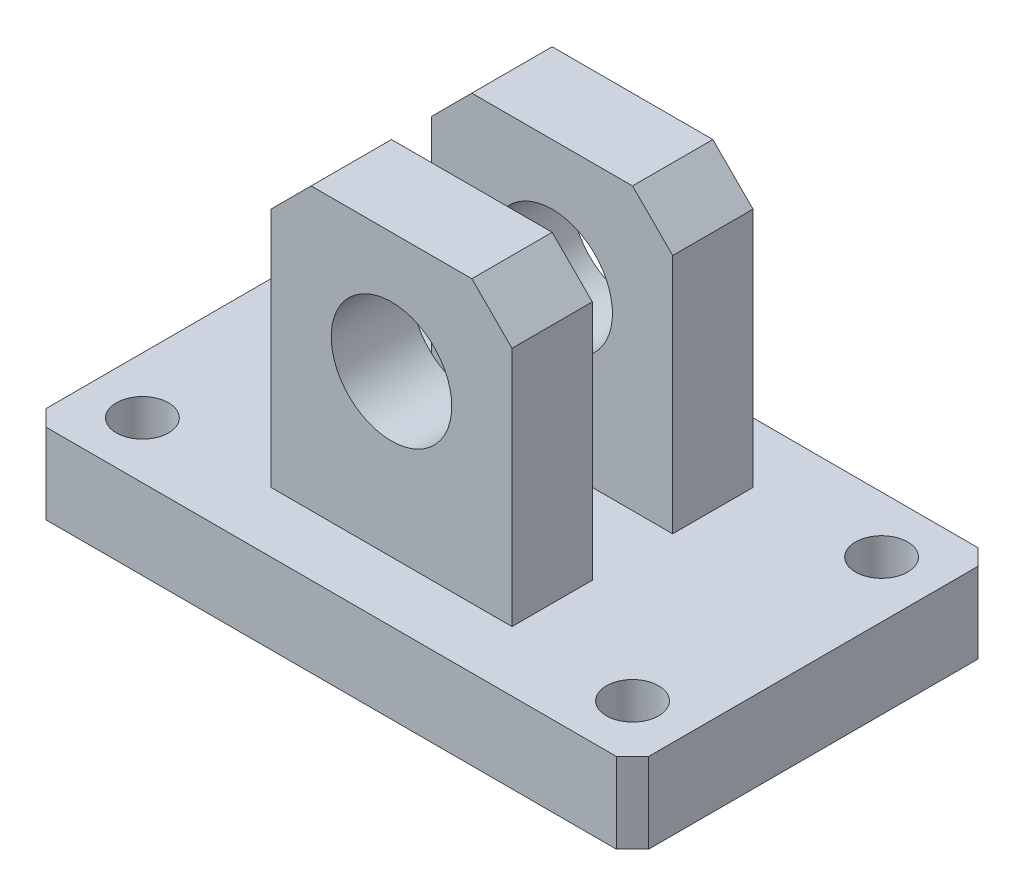
ISO-10303-21;
HEADER;
FILE_DESCRIPTION(('STEP AP214'),'2;1');
FILE_NAME('part.step','',(''),(''),'','','');
FILE_SCHEMA(('AUTOMOTIVE_DESIGN { 1 0 10303 214 1 1 1 1 }'));
ENDSEC;
DATA;
#1=APPLICATION_CONTEXT('core data for automotive mechanical design processes');
#2=APPLICATION_PROTOCOL_DEFINITION('international standard','automotive_design',2000,#1);
#3=PRODUCT_CONTEXT('',#1,'mechanical');
#4=PRODUCT('Part','Part','',(#3));
#5=PRODUCT_RELATED_PRODUCT_CATEGORY('part','',(#4));
#6=PRODUCT_DEFINITION_FORMATION('','',#4);
#7=PRODUCT_DEFINITION_CONTEXT('part definition',#1,'design');
#8=PRODUCT_DEFINITION('design','',#6,#7);
#9=PRODUCT_DEFINITION_SHAPE('','',#8);
#10=(LENGTH_UNIT() NAMED_UNIT(*) SI_UNIT(.MILLI.,.METRE.));
#11=(NAMED_UNIT(*) PLANE_ANGLE_UNIT() SI_UNIT($,.RADIAN.));
#12=(NAMED_UNIT(*) SI_UNIT($,.STERADIAN.) SOLID_ANGLE_UNIT());
#13=UNCERTAINTY_MEASURE_WITH_UNIT(LENGTH_MEASURE(1.E-05),#10,'distance_accuracy_value','');
#14=(GEOMETRIC_REPRESENTATION_CONTEXT(3) GLOBAL_UNCERTAINTY_ASSIGNED_CONTEXT((#13)) GLOBAL_UNIT_ASSIGNED_CONTEXT((#10,
#11,#12)) REPRESENTATION_CONTEXT('',''));
#15=CARTESIAN_POINT('',(0.,0.,0.));
#16=DIRECTION('',(0.,0.,1.));
#17=DIRECTION('',(1.,0.,0.));
#18=AXIS2_PLACEMENT_3D('',#15,#16,#17);
#19=CARTESIAN_POINT('',(0.,10.,0.));
#20=DIRECTION('',(0.,-1.,0.));
#21=DIRECTION('',(0.,0.,-1.));
#22=AXIS2_PLACEMENT_3D('',#19,#20,#21);
#23=PLANE('',#22);
#24=CARTESIAN_POINT('',(30.5,10.,-15.5));
#25=DIRECTION('',(0.,1.,0.));
#26=DIRECTION('',(0.,0.,-1.));
#27=AXIS2_PLACEMENT_3D('',#24,#25,#26);
#28=CIRCLE('',#27,3.25000000000002);
#29=CARTESIAN_POINT('',(30.5,10.,-18.75));
#30=VERTEX_POINT('',#29);
#31=EDGE_CURVE('E532',#30,#30,#28,.T.);
#32=ORIENTED_EDGE('',*,*,#31,.F.);
#33=EDGE_LOOP('',(#32));
#34=FACE_BOUND('',#33,.T.);
#35=CARTESIAN_POINT('',(30.5,10.,15.5));
#36=DIRECTION('',(0.,1.,0.));
#37=DIRECTION('',(0.,0.,-1.));
#38=AXIS2_PLACEMENT_3D('',#35,#36,#37);
#39=CIRCLE('',#38,3.25000000000002);
#40=CARTESIAN_POINT('',(30.5,10.,12.25));
#41=VERTEX_POINT('',#40);
#42=EDGE_CURVE('E522',#41,#41,#39,.T.);
#43=ORIENTED_EDGE('',*,*,#42,.F.);
#44=EDGE_LOOP('',(#43));
#45=FACE_BOUND('',#44,.T.);
#46=CARTESIAN_POINT('',(-30.5,10.,15.5));
#47=DIRECTION('',(0.,1.,0.));
#48=DIRECTION('',(0.,0.,1.));
#49=AXIS2_PLACEMENT_3D('',#46,#47,#48);
#50=CIRCLE('',#49,3.25);
#51=CARTESIAN_POINT('',(-30.5,10.,18.75));
#52=VERTEX_POINT('',#51);
#53=EDGE_CURVE('E517',#52,#52,#50,.T.);
#54=ORIENTED_EDGE('',*,*,#53,.F.);
#55=EDGE_LOOP('',(#54));
#56=FACE_BOUND('',#55,.T.);
#57=CARTESIAN_POINT('',(-30.5,10.,-15.5));
#58=DIRECTION('',(0.,1.,0.));
#59=DIRECTION('',(0.,0.,1.));
#60=AXIS2_PLACEMENT_3D('',#57,#58,#59);
#61=CIRCLE('',#60,3.25);
#62=CARTESIAN_POINT('',(-30.5,10.,-12.25));
#63=VERTEX_POINT('',#62);
#64=EDGE_CURVE('E518',#63,#63,#61,.T.);
#65=ORIENTED_EDGE('',*,*,#64,.F.);
#66=EDGE_LOOP('',(#65));
#67=FACE_BOUND('',#66,.T.);
#68=DIRECTION('',(-1.,0.,0.));
#69=VECTOR('',#68,1.);
#70=CARTESIAN_POINT('',(-37.5,10.,-22.5));
#71=LINE('',#70,#69);
#72=CARTESIAN_POINT('',(35.5,10.,-22.5));
#73=VERTEX_POINT('',#72);
#74=CARTESIAN_POINT('',(-35.5,10.,-22.5));
#75=VERTEX_POINT('',#74);
#76=EDGE_CURVE('E237',#73,#75,#71,.T.);
#77=ORIENTED_EDGE('',*,*,#76,.T.);
#78=DIRECTION('',(0.707106781186549,0.,-0.707106781186546));
#79=VECTOR('',#78,1.);
#80=CARTESIAN_POINT('',(-37.5,10.,-20.5));
#81=LINE('',#80,#79);
#82=CARTESIAN_POINT('',(-37.5,10.,-20.5));
#83=VERTEX_POINT('',#82);
#84=EDGE_CURVE('E283',#75,#83,#81,.F.);
#85=ORIENTED_EDGE('',*,*,#84,.T.);
#86=DIRECTION('',(0.,0.,1.));
#87=VECTOR('',#86,1.);
#88=CARTESIAN_POINT('',(-37.5,10.,22.5));
#89=LINE('',#88,#87);
#90=CARTESIAN_POINT('',(-37.5,10.,20.5));
#91=VERTEX_POINT('',#90);
#92=EDGE_CURVE('E245',#83,#91,#89,.T.);
#93=ORIENTED_EDGE('',*,*,#92,.T.);
#94=DIRECTION('',(-0.707106781186546,0.,-0.707106781186549));
#95=VECTOR('',#94,1.);
#96=CARTESIAN_POINT('',(-35.5,10.,22.5));
#97=LINE('',#96,#95);
#98=CARTESIAN_POINT('',(-35.5,10.,22.5));
#99=VERTEX_POINT('',#98);
#100=EDGE_CURVE('E271',#91,#99,#97,.F.);
#101=ORIENTED_EDGE('',*,*,#100,.T.);
#102=DIRECTION('',(1.,0.,0.));
#103=VECTOR('',#102,1.);
#104=CARTESIAN_POINT('',(-37.5,10.,22.5));
#105=LINE('',#104,#103);
#106=CARTESIAN_POINT('',(35.5,10.,22.5));
#107=VERTEX_POINT('',#106);
#108=EDGE_CURVE('E242',#99,#107,#105,.T.);
#109=ORIENTED_EDGE('',*,*,#108,.T.);
#110=DIRECTION('',(-0.707106781186548,0.,0.707106781186548));
#111=VECTOR('',#110,1.);
#112=CARTESIAN_POINT('',(37.5,10.,20.5));
#113=LINE('',#112,#111);
#114=CARTESIAN_POINT('',(37.5,10.,20.5));
#115=VERTEX_POINT('',#114);
#116=EDGE_CURVE('E265',#107,#115,#113,.F.);
#117=ORIENTED_EDGE('',*,*,#116,.T.);
#118=DIRECTION('',(0.,0.,-1.));
#119=VECTOR('',#118,1.);
#120=CARTESIAN_POINT('',(37.5,10.,22.5));
#121=LINE('',#120,#119);
#122=CARTESIAN_POINT('',(37.5,10.,-20.5));
#123=VERTEX_POINT('',#122);
#124=EDGE_CURVE('E236',#115,#123,#121,.T.);
#125=ORIENTED_EDGE('',*,*,#124,.T.);
#126=DIRECTION('',(0.707106781186546,0.,0.707106781186549));
#127=VECTOR('',#126,1.);
#128=CARTESIAN_POINT('',(35.5,10.,-22.5));
#129=LINE('',#128,#127);
#130=EDGE_CURVE('E291',#123,#73,#129,.F.);
#131=ORIENTED_EDGE('',*,*,#130,.T.);
#132=EDGE_LOOP('',(#77,#85,#93,#101,#109,#117,#125,#131));
#133=FACE_BOUND('',#132,.T.);
#134=DIRECTION('',(-1.,0.,0.));
#135=VECTOR('',#134,1.);
#136=CARTESIAN_POINT('',(-15.,10.,-15.));
#137=LINE('',#136,#135);
#138=CARTESIAN_POINT('',(15.,10.,-15.));
#139=VERTEX_POINT('',#138);
#140=CARTESIAN_POINT('',(-15.,10.,-15.));
#141=VERTEX_POINT('',#140);
#142=EDGE_CURVE('E178',#139,#141,#137,.T.);
#143=ORIENTED_EDGE('',*,*,#142,.F.);
#144=DIRECTION('',(0.,0.,-1.));
#145=VECTOR('',#144,1.);
#146=CARTESIAN_POINT('',(15.,10.,-4.99999999999999));
#147=LINE('',#146,#145);
#148=CARTESIAN_POINT('',(15.,10.,-4.99999999999999));
#149=VERTEX_POINT('',#148);
#150=EDGE_CURVE('E189',#149,#139,#147,.T.);
#151=ORIENTED_EDGE('',*,*,#150,.F.);
#152=DIRECTION('',(-1.,0.,0.));
#153=VECTOR('',#152,1.);
#154=CARTESIAN_POINT('',(-15.,10.,-4.99999999999999));
#155=LINE('',#154,#153);
#156=CARTESIAN_POINT('',(-15.,10.,-4.99999999999999));
#157=VERTEX_POINT('',#156);
#158=EDGE_CURVE('E338',#149,#157,#155,.T.);
#159=ORIENTED_EDGE('',*,*,#158,.T.);
#160=DIRECTION('',(0.,0.,-1.));
#161=VECTOR('',#160,1.);
#162=CARTESIAN_POINT('',(-15.,10.,-4.99999999999999));
#163=LINE('',#162,#161);
#164=EDGE_CURVE('E192',#157,#141,#163,.T.);
#165=ORIENTED_EDGE('',*,*,#164,.T.);
#166=EDGE_LOOP('',(#143,#151,#159,#165));
#167=FACE_BOUND('',#166,.T.);
#168=DIRECTION('',(0.,0.,-1.));
#169=VECTOR('',#168,1.);
#170=CARTESIAN_POINT('',(15.,10.,15.));
#171=LINE('',#170,#169);
#172=CARTESIAN_POINT('',(15.,10.,15.));
#173=VERTEX_POINT('',#172);
#174=CARTESIAN_POINT('',(15.,10.,5.));
#175=VERTEX_POINT('',#174);
#176=EDGE_CURVE('E221',#173,#175,#171,.T.);
#177=ORIENTED_EDGE('',*,*,#176,.F.);
#178=DIRECTION('',(1.,0.,0.));
#179=VECTOR('',#178,1.);
#180=CARTESIAN_POINT('',(-15.,10.,15.));
#181=LINE('',#180,#179);
#182=CARTESIAN_POINT('',(-15.,10.,15.));
#183=VERTEX_POINT('',#182);
#184=EDGE_CURVE('E217',#183,#173,#181,.T.);
#185=ORIENTED_EDGE('',*,*,#184,.F.);
#186=DIRECTION('',(0.,0.,-1.));
#187=VECTOR('',#186,1.);
#188=CARTESIAN_POINT('',(-15.,10.,15.));
#189=LINE('',#188,#187);
#190=CARTESIAN_POINT('',(-15.,10.,5.));
#191=VERTEX_POINT('',#190);
#192=EDGE_CURVE('E235',#183,#191,#189,.T.);
#193=ORIENTED_EDGE('',*,*,#192,.T.);
#194=DIRECTION('',(1.,0.,0.));
#195=VECTOR('',#194,1.);
#196=CARTESIAN_POINT('',(-15.,10.,5.));
#197=LINE('',#196,#195);
#198=EDGE_CURVE('E214',#191,#175,#197,.T.);
#199=ORIENTED_EDGE('',*,*,#198,.T.);
#200=EDGE_LOOP('',(#177,#185,#193,#199));
#201=FACE_BOUND('',#200,.T.);
#202=ADVANCED_FACE('F41',(#34,#45,#56,#67,#133,#167,#201),#23,.F.);
#203=CARTESIAN_POINT('',(37.5,10.,22.5));
#204=DIRECTION('',(-1.,0.,0.));
#205=DIRECTION('',(0.,0.,1.));
#206=AXIS2_PLACEMENT_3D('',#203,#204,#205);
#207=PLANE('',#206);
#208=DIRECTION('',(0.,0.,-1.));
#209=VECTOR('',#208,1.);
#210=CARTESIAN_POINT('',(37.5,0.,22.5));
#211=LINE('',#210,#209);
#212=CARTESIAN_POINT('',(37.5,0.,20.5));
#213=VERTEX_POINT('',#212);
#214=CARTESIAN_POINT('',(37.5,0.,-20.5));
#215=VERTEX_POINT('',#214);
#216=EDGE_CURVE('E232',#213,#215,#211,.T.);
#217=ORIENTED_EDGE('',*,*,#216,.T.);
#218=DIRECTION('',(0.,1.,0.));
#219=VECTOR('',#218,1.);
#220=CARTESIAN_POINT('',(37.5,10.,-20.5));
#221=LINE('',#220,#219);
#222=EDGE_CURVE('E293',#215,#123,#221,.T.);
#223=ORIENTED_EDGE('',*,*,#222,.T.);
#224=ORIENTED_EDGE('',*,*,#124,.F.);
#225=DIRECTION('',(0.,-1.,0.));
#226=VECTOR('',#225,1.);
#227=CARTESIAN_POINT('',(37.5,10.,20.5));
#228=LINE('',#227,#226);
#229=EDGE_CURVE('E246',#115,#213,#228,.T.);
#230=ORIENTED_EDGE('',*,*,#229,.T.);
#231=EDGE_LOOP('',(#217,#223,#224,#230));
#232=FACE_BOUND('',#231,.T.);
#233=ADVANCED_FACE('F366',(#232),#207,.F.);
#234=CARTESIAN_POINT('',(-37.5,10.,-22.5));
#235=DIRECTION('',(0.,0.,1.));
#236=DIRECTION('',(1.,0.,0.));
#237=AXIS2_PLACEMENT_3D('',#234,#235,#236);
#238=PLANE('',#237);
#239=DIRECTION('',(0.,1.,0.));
#240=VECTOR('',#239,1.);
#241=CARTESIAN_POINT('',(-35.5,10.,-22.5));
#242=LINE('',#241,#240);
#243=CARTESIAN_POINT('',(-35.5,0.,-22.5));
#244=VERTEX_POINT('',#243);
#245=EDGE_CURVE('E281',#244,#75,#242,.T.);
#246=ORIENTED_EDGE('',*,*,#245,.T.);
#247=ORIENTED_EDGE('',*,*,#76,.F.);
#248=DIRECTION('',(0.,-1.,0.));
#249=VECTOR('',#248,1.);
#250=CARTESIAN_POINT('',(35.5,10.,-22.5));
#251=LINE('',#250,#249);
#252=CARTESIAN_POINT('',(35.5,0.,-22.5));
#253=VERTEX_POINT('',#252);
#254=EDGE_CURVE('E286',#73,#253,#251,.T.);
#255=ORIENTED_EDGE('',*,*,#254,.T.);
#256=DIRECTION('',(-1.,0.,0.));
#257=VECTOR('',#256,1.);
#258=CARTESIAN_POINT('',(-37.5,0.,-22.5));
#259=LINE('',#258,#257);
#260=EDGE_CURVE('E248',#253,#244,#259,.T.);
#261=ORIENTED_EDGE('',*,*,#260,.T.);
#262=EDGE_LOOP('',(#246,#247,#255,#261));
#263=FACE_BOUND('',#262,.T.);
#264=ADVANCED_FACE('F373',(#263),#238,.F.);
#265=CARTESIAN_POINT('',(-37.5,10.,22.5));
#266=DIRECTION('',(1.,0.,0.));
#267=DIRECTION('',(0.,0.,-1.));
#268=AXIS2_PLACEMENT_3D('',#265,#266,#267);
#269=PLANE('',#268);
#270=ORIENTED_EDGE('',*,*,#92,.F.);
#271=DIRECTION('',(0.,-1.,0.));
#272=VECTOR('',#271,1.);
#273=CARTESIAN_POINT('',(-37.5,10.,-20.5));
#274=LINE('',#273,#272);
#275=CARTESIAN_POINT('',(-37.5,0.,-20.5));
#276=VERTEX_POINT('',#275);
#277=EDGE_CURVE('E273',#83,#276,#274,.T.);
#278=ORIENTED_EDGE('',*,*,#277,.T.);
#279=DIRECTION('',(0.,0.,1.));
#280=VECTOR('',#279,1.);
#281=CARTESIAN_POINT('',(-37.5,0.,22.5));
#282=LINE('',#281,#280);
#283=CARTESIAN_POINT('',(-37.5,0.,20.5));
#284=VERTEX_POINT('',#283);
#285=EDGE_CURVE('E252',#276,#284,#282,.T.);
#286=ORIENTED_EDGE('',*,*,#285,.T.);
#287=DIRECTION('',(0.,1.,0.));
#288=VECTOR('',#287,1.);
#289=CARTESIAN_POINT('',(-37.5,10.,20.5));
#290=LINE('',#289,#288);
#291=EDGE_CURVE('E270',#284,#91,#290,.T.);
#292=ORIENTED_EDGE('',*,*,#291,.T.);
#293=EDGE_LOOP('',(#270,#278,#286,#292));
#294=FACE_BOUND('',#293,.T.);
#295=ADVANCED_FACE('F386',(#294),#269,.F.);
#296=CARTESIAN_POINT('',(-37.5,10.,22.5));
#297=DIRECTION('',(0.,0.,-1.));
#298=DIRECTION('',(-1.,0.,0.));
#299=AXIS2_PLACEMENT_3D('',#296,#297,#298);
#300=PLANE('',#299);
#301=ORIENTED_EDGE('',*,*,#108,.F.);
#302=DIRECTION('',(0.,-1.,0.));
#303=VECTOR('',#302,1.);
#304=CARTESIAN_POINT('',(-35.5,10.,22.5));
#305=LINE('',#304,#303);
#306=CARTESIAN_POINT('',(-35.5,0.,22.5));
#307=VERTEX_POINT('',#306);
#308=EDGE_CURVE('E263',#99,#307,#305,.T.);
#309=ORIENTED_EDGE('',*,*,#308,.T.);
#310=DIRECTION('',(1.,0.,0.));
#311=VECTOR('',#310,1.);
#312=CARTESIAN_POINT('',(-37.5,0.,22.5));
#313=LINE('',#312,#311);
#314=CARTESIAN_POINT('',(35.5,0.,22.5));
#315=VERTEX_POINT('',#314);
#316=EDGE_CURVE('E239',#307,#315,#313,.T.);
#317=ORIENTED_EDGE('',*,*,#316,.T.);
#318=DIRECTION('',(0.,1.,0.));
#319=VECTOR('',#318,1.);
#320=CARTESIAN_POINT('',(35.5,10.,22.5));
#321=LINE('',#320,#319);
#322=EDGE_CURVE('E256',#315,#107,#321,.T.);
#323=ORIENTED_EDGE('',*,*,#322,.T.);
#324=EDGE_LOOP('',(#301,#309,#317,#323));
#325=FACE_BOUND('',#324,.T.);
#326=ADVANCED_FACE('F383',(#325),#300,.F.);
#327=CARTESIAN_POINT('',(0.,0.,0.));
#328=DIRECTION('',(0.,-1.,0.));
#329=DIRECTION('',(0.,0.,-1.));
#330=AXIS2_PLACEMENT_3D('',#327,#328,#329);
#331=PLANE('',#330);
#332=CARTESIAN_POINT('',(30.5,0.,-15.5));
#333=DIRECTION('',(0.,1.,0.));
#334=DIRECTION('',(0.,0.,-1.));
#335=AXIS2_PLACEMENT_3D('',#332,#333,#334);
#336=CIRCLE('',#335,3.25000000000002);
#337=CARTESIAN_POINT('',(30.5,0.,-18.75));
#338=VERTEX_POINT('',#337);
#339=EDGE_CURVE('E529',#338,#338,#336,.T.);
#340=ORIENTED_EDGE('',*,*,#339,.T.);
#341=EDGE_LOOP('',(#340));
#342=FACE_BOUND('',#341,.T.);
#343=CARTESIAN_POINT('',(30.5,0.,15.5));
#344=DIRECTION('',(0.,1.,0.));
#345=DIRECTION('',(0.,0.,-1.));
#346=AXIS2_PLACEMENT_3D('',#343,#344,#345);
#347=CIRCLE('',#346,3.25000000000002);
#348=CARTESIAN_POINT('',(30.5,0.,12.25));
#349=VERTEX_POINT('',#348);
#350=EDGE_CURVE('E519',#349,#349,#347,.T.);
#351=ORIENTED_EDGE('',*,*,#350,.T.);
#352=EDGE_LOOP('',(#351));
#353=FACE_BOUND('',#352,.T.);
#354=CARTESIAN_POINT('',(-30.5,0.,15.5));
#355=DIRECTION('',(0.,1.,0.));
#356=DIRECTION('',(0.,0.,1.));
#357=AXIS2_PLACEMENT_3D('',#354,#355,#356);
#358=CIRCLE('',#357,3.25);
#359=CARTESIAN_POINT('',(-30.5,0.,18.75));
#360=VERTEX_POINT('',#359);
#361=EDGE_CURVE('E514',#360,#360,#358,.T.);
#362=ORIENTED_EDGE('',*,*,#361,.T.);
#363=EDGE_LOOP('',(#362));
#364=FACE_BOUND('',#363,.T.);
#365=CARTESIAN_POINT('',(-30.5,0.,-15.5));
#366=DIRECTION('',(0.,1.,0.));
#367=DIRECTION('',(0.,0.,1.));
#368=AXIS2_PLACEMENT_3D('',#365,#366,#367);
#369=CIRCLE('',#368,3.25);
#370=CARTESIAN_POINT('',(-30.5,0.,-12.25));
#371=VERTEX_POINT('',#370);
#372=EDGE_CURVE('E534',#371,#371,#369,.T.);
#373=ORIENTED_EDGE('',*,*,#372,.T.);
#374=EDGE_LOOP('',(#373));
#375=FACE_BOUND('',#374,.T.);
#376=ORIENTED_EDGE('',*,*,#260,.F.);
#377=DIRECTION('',(-0.707106781186546,0.,-0.707106781186549));
#378=VECTOR('',#377,1.);
#379=CARTESIAN_POINT('',(29.0000000000001,0.,-29.));
#380=LINE('',#379,#378);
#381=EDGE_CURVE('E288',#253,#215,#380,.F.);
#382=ORIENTED_EDGE('',*,*,#381,.T.);
#383=ORIENTED_EDGE('',*,*,#216,.F.);
#384=DIRECTION('',(0.707106781186548,0.,-0.707106781186548));
#385=VECTOR('',#384,1.);
#386=CARTESIAN_POINT('',(29.,0.,29.));
#387=LINE('',#386,#385);
#388=EDGE_CURVE('E257',#213,#315,#387,.F.);
#389=ORIENTED_EDGE('',*,*,#388,.T.);
#390=ORIENTED_EDGE('',*,*,#316,.F.);
#391=DIRECTION('',(0.707106781186546,0.,0.707106781186549));
#392=VECTOR('',#391,1.);
#393=CARTESIAN_POINT('',(-29.0000000000001,0.,29.));
#394=LINE('',#393,#392);
#395=EDGE_CURVE('E267',#307,#284,#394,.F.);
#396=ORIENTED_EDGE('',*,*,#395,.T.);
#397=ORIENTED_EDGE('',*,*,#285,.F.);
#398=DIRECTION('',(-0.707106781186549,0.,0.707106781186546));
#399=VECTOR('',#398,1.);
#400=CARTESIAN_POINT('',(-28.9999999999999,0.,-29.));
#401=LINE('',#400,#399);
#402=EDGE_CURVE('E279',#276,#244,#401,.F.);
#403=ORIENTED_EDGE('',*,*,#402,.T.);
#404=EDGE_LOOP('',(#376,#382,#383,#389,#390,#396,#397,#403));
#405=FACE_BOUND('',#404,.T.);
#406=ADVANCED_FACE('F385',(#342,#353,#364,#375,#405),#331,.T.);
#407=CARTESIAN_POINT('',(37.5,10.,20.5));
#408=DIRECTION('',(-0.707106781186547,0.,-0.707106781186547));
#409=DIRECTION('',(0.,-1.,0.));
#410=AXIS2_PLACEMENT_3D('',#407,#408,#409);
#411=PLANE('',#410);
#412=ORIENTED_EDGE('',*,*,#116,.F.);
#413=ORIENTED_EDGE('',*,*,#322,.F.);
#414=ORIENTED_EDGE('',*,*,#388,.F.);
#415=ORIENTED_EDGE('',*,*,#229,.F.);
#416=EDGE_LOOP('',(#412,#413,#414,#415));
#417=FACE_BOUND('',#416,.T.);
#418=ADVANCED_FACE('F381',(#417),#411,.F.);
#419=CARTESIAN_POINT('',(-35.5,10.,22.5));
#420=DIRECTION('',(0.707106781186549,0.,-0.707106781186546));
#421=DIRECTION('',(0.,-1.,0.));
#422=AXIS2_PLACEMENT_3D('',#419,#420,#421);
#423=PLANE('',#422);
#424=ORIENTED_EDGE('',*,*,#100,.F.);
#425=ORIENTED_EDGE('',*,*,#291,.F.);
#426=ORIENTED_EDGE('',*,*,#395,.F.);
#427=ORIENTED_EDGE('',*,*,#308,.F.);
#428=EDGE_LOOP('',(#424,#425,#426,#427));
#429=FACE_BOUND('',#428,.T.);
#430=ADVANCED_FACE('F401',(#429),#423,.F.);
#431=CARTESIAN_POINT('',(-37.5,10.,-20.5));
#432=DIRECTION('',(0.707106781186546,0.,0.707106781186549));
#433=DIRECTION('',(0.,-1.,0.));
#434=AXIS2_PLACEMENT_3D('',#431,#432,#433);
#435=PLANE('',#434);
#436=ORIENTED_EDGE('',*,*,#84,.F.);
#437=ORIENTED_EDGE('',*,*,#245,.F.);
#438=ORIENTED_EDGE('',*,*,#402,.F.);
#439=ORIENTED_EDGE('',*,*,#277,.F.);
#440=EDGE_LOOP('',(#436,#437,#438,#439));
#441=FACE_BOUND('',#440,.T.);
#442=ADVANCED_FACE('F408',(#441),#435,.F.);
#443=CARTESIAN_POINT('',(35.5,10.,-22.5));
#444=DIRECTION('',(-0.707106781186549,0.,0.707106781186546));
#445=DIRECTION('',(0.,-1.,0.));
#446=AXIS2_PLACEMENT_3D('',#443,#444,#445);
#447=PLANE('',#446);
#448=ORIENTED_EDGE('',*,*,#130,.F.);
#449=ORIENTED_EDGE('',*,*,#222,.F.);
#450=ORIENTED_EDGE('',*,*,#381,.F.);
#451=ORIENTED_EDGE('',*,*,#254,.F.);
#452=EDGE_LOOP('',(#448,#449,#450,#451));
#453=FACE_BOUND('',#452,.T.);
#454=ADVANCED_FACE('F417',(#453),#447,.F.);
#455=CARTESIAN_POINT('',(0.,0.,15.));
#456=DIRECTION('',(0.,0.,1.));
#457=DIRECTION('',(1.,0.,0.));
#458=AXIS2_PLACEMENT_3D('',#455,#456,#457);
#459=PLANE('',#458);
#460=DIRECTION('',(-1.,0.,0.));
#461=VECTOR('',#460,1.);
#462=CARTESIAN_POINT('',(-15.,45.,15.));
#463=LINE('',#462,#461);
#464=CARTESIAN_POINT('',(9.99999999999997,45.,15.));
#465=VERTEX_POINT('',#464);
#466=CARTESIAN_POINT('',(-10.,45.,15.));
#467=VERTEX_POINT('',#466);
#468=EDGE_CURVE('E215',#465,#467,#463,.T.);
#469=ORIENTED_EDGE('',*,*,#468,.T.);
#470=DIRECTION('',(0.70710678118655,0.707106781186546,0.));
#471=VECTOR('',#470,1.);
#472=CARTESIAN_POINT('',(-27.5,27.5000000000001,15.));
#473=LINE('',#472,#471);
#474=CARTESIAN_POINT('',(-15.,40.,15.));
#475=VERTEX_POINT('',#474);
#476=EDGE_CURVE('E319',#467,#475,#473,.F.);
#477=ORIENTED_EDGE('',*,*,#476,.T.);
#478=DIRECTION('',(0.,-1.,0.));
#479=VECTOR('',#478,1.);
#480=CARTESIAN_POINT('',(-15.,10.,15.));
#481=LINE('',#480,#479);
#482=EDGE_CURVE('E216',#475,#183,#481,.T.);
#483=ORIENTED_EDGE('',*,*,#482,.T.);
#484=ORIENTED_EDGE('',*,*,#184,.T.);
#485=DIRECTION('',(0.,1.,0.));
#486=VECTOR('',#485,1.);
#487=CARTESIAN_POINT('',(15.,45.,15.));
#488=LINE('',#487,#486);
#489=CARTESIAN_POINT('',(15.,40.,15.));
#490=VERTEX_POINT('',#489);
#491=EDGE_CURVE('E209',#173,#490,#488,.T.);
#492=ORIENTED_EDGE('',*,*,#491,.T.);
#493=DIRECTION('',(0.707106781186547,-0.707106781186549,0.));
#494=VECTOR('',#493,1.);
#495=CARTESIAN_POINT('',(27.5,27.4999999999999,15.));
#496=LINE('',#495,#494);
#497=EDGE_CURVE('E317',#490,#465,#496,.F.);
#498=ORIENTED_EDGE('',*,*,#497,.T.);
#499=EDGE_LOOP('',(#469,#477,#483,#484,#492,#498));
#500=FACE_BOUND('',#499,.T.);
#501=CARTESIAN_POINT('',(0.,30.,15.));
#502=DIRECTION('',(0.,0.,1.));
#503=DIRECTION('',(1.,0.,0.));
#504=AXIS2_PLACEMENT_3D('',#501,#502,#503);
#505=CIRCLE('',#504,7.5);
#506=CARTESIAN_POINT('',(7.49999999999997,30.,15.));
#507=VERTEX_POINT('',#506);
#508=EDGE_CURVE('E199',#507,#507,#505,.T.);
#509=ORIENTED_EDGE('',*,*,#508,.F.);
#510=EDGE_LOOP('',(#509));
#511=FACE_BOUND('',#510,.T.);
#512=ADVANCED_FACE('F425',(#500,#511),#459,.T.);
#513=CARTESIAN_POINT('',(0.,0.,5.));
#514=DIRECTION('',(0.,0.,1.));
#515=DIRECTION('',(1.,0.,0.));
#516=AXIS2_PLACEMENT_3D('',#513,#514,#515);
#517=PLANE('',#516);
#518=DIRECTION('',(0.,-1.,0.));
#519=VECTOR('',#518,1.);
#520=CARTESIAN_POINT('',(-15.,10.,5.));
#521=LINE('',#520,#519);
#522=CARTESIAN_POINT('',(-15.,40.,5.));
#523=VERTEX_POINT('',#522);
#524=EDGE_CURVE('E227',#523,#191,#521,.T.);
#525=ORIENTED_EDGE('',*,*,#524,.F.);
#526=DIRECTION('',(-0.70710678118655,-0.707106781186546,0.));
#527=VECTOR('',#526,1.);
#528=CARTESIAN_POINT('',(-15.,40.,5.));
#529=LINE('',#528,#527);
#530=CARTESIAN_POINT('',(-10.,45.,5.));
#531=VERTEX_POINT('',#530);
#532=EDGE_CURVE('E307',#523,#531,#529,.F.);
#533=ORIENTED_EDGE('',*,*,#532,.T.);
#534=DIRECTION('',(-1.,0.,0.));
#535=VECTOR('',#534,1.);
#536=CARTESIAN_POINT('',(-15.,45.,5.));
#537=LINE('',#536,#535);
#538=CARTESIAN_POINT('',(9.99999999999997,45.,5.));
#539=VERTEX_POINT('',#538);
#540=EDGE_CURVE('E223',#539,#531,#537,.T.);
#541=ORIENTED_EDGE('',*,*,#540,.F.);
#542=DIRECTION('',(-0.707106781186547,0.707106781186549,0.));
#543=VECTOR('',#542,1.);
#544=CARTESIAN_POINT('',(9.99999999999997,45.,5.));
#545=LINE('',#544,#543);
#546=CARTESIAN_POINT('',(15.,40.,5.));
#547=VERTEX_POINT('',#546);
#548=EDGE_CURVE('E310',#539,#547,#545,.F.);
#549=ORIENTED_EDGE('',*,*,#548,.T.);
#550=DIRECTION('',(0.,1.,0.));
#551=VECTOR('',#550,1.);
#552=CARTESIAN_POINT('',(15.,45.,5.));
#553=LINE('',#552,#551);
#554=EDGE_CURVE('E210',#175,#547,#553,.T.);
#555=ORIENTED_EDGE('',*,*,#554,.F.);
#556=ORIENTED_EDGE('',*,*,#198,.F.);
#557=EDGE_LOOP('',(#525,#533,#541,#549,#555,#556));
#558=FACE_BOUND('',#557,.T.);
#559=CARTESIAN_POINT('',(0.,30.,5.));
#560=DIRECTION('',(0.,0.,1.));
#561=DIRECTION('',(1.,0.,0.));
#562=AXIS2_PLACEMENT_3D('',#559,#560,#561);
#563=CIRCLE('',#562,7.5);
#564=CARTESIAN_POINT('',(7.49999999999997,30.,5.));
#565=VERTEX_POINT('',#564);
#566=EDGE_CURVE('E200',#565,#565,#563,.T.);
#567=ORIENTED_EDGE('',*,*,#566,.T.);
#568=EDGE_LOOP('',(#567));
#569=FACE_BOUND('',#568,.T.);
#570=ADVANCED_FACE('F457',(#558,#569),#517,.F.);
#571=CARTESIAN_POINT('',(15.,45.,15.));
#572=DIRECTION('',(-1.,0.,0.));
#573=DIRECTION('',(0.,0.,1.));
#574=AXIS2_PLACEMENT_3D('',#571,#572,#573);
#575=PLANE('',#574);
#576=ORIENTED_EDGE('',*,*,#554,.T.);
#577=DIRECTION('',(0.,0.,1.));
#578=VECTOR('',#577,1.);
#579=CARTESIAN_POINT('',(15.,40.,15.));
#580=LINE('',#579,#578);
#581=EDGE_CURVE('E318',#547,#490,#580,.T.);
#582=ORIENTED_EDGE('',*,*,#581,.T.);
#583=ORIENTED_EDGE('',*,*,#491,.F.);
#584=ORIENTED_EDGE('',*,*,#176,.T.);
#585=EDGE_LOOP('',(#576,#582,#583,#584));
#586=FACE_BOUND('',#585,.T.);
#587=ADVANCED_FACE('F379',(#586),#575,.F.);
#588=CARTESIAN_POINT('',(-15.,45.,15.));
#589=DIRECTION('',(0.,-1.,0.));
#590=DIRECTION('',(0.,0.,-1.));
#591=AXIS2_PLACEMENT_3D('',#588,#589,#590);
#592=PLANE('',#591);
#593=ORIENTED_EDGE('',*,*,#540,.T.);
#594=DIRECTION('',(0.,0.,1.));
#595=VECTOR('',#594,1.);
#596=CARTESIAN_POINT('',(-10.,45.,15.));
#597=LINE('',#596,#595);
#598=EDGE_CURVE('E313',#531,#467,#597,.T.);
#599=ORIENTED_EDGE('',*,*,#598,.T.);
#600=ORIENTED_EDGE('',*,*,#468,.F.);
#601=DIRECTION('',(0.,0.,-1.));
#602=VECTOR('',#601,1.);
#603=CARTESIAN_POINT('',(9.99999999999997,45.,15.));
#604=LINE('',#603,#602);
#605=EDGE_CURVE('E311',#465,#539,#604,.T.);
#606=ORIENTED_EDGE('',*,*,#605,.T.);
#607=EDGE_LOOP('',(#593,#599,#600,#606));
#608=FACE_BOUND('',#607,.T.);
#609=ADVANCED_FACE('F470',(#608),#592,.F.);
#610=CARTESIAN_POINT('',(-15.,10.,15.));
#611=DIRECTION('',(1.,0.,0.));
#612=DIRECTION('',(0.,0.,-1.));
#613=AXIS2_PLACEMENT_3D('',#610,#611,#612);
#614=PLANE('',#613);
#615=ORIENTED_EDGE('',*,*,#482,.F.);
#616=DIRECTION('',(0.,0.,-1.));
#617=VECTOR('',#616,1.);
#618=CARTESIAN_POINT('',(-15.,40.,15.));
#619=LINE('',#618,#617);
#620=EDGE_CURVE('E302',#475,#523,#619,.T.);
#621=ORIENTED_EDGE('',*,*,#620,.T.);
#622=ORIENTED_EDGE('',*,*,#524,.T.);
#623=ORIENTED_EDGE('',*,*,#192,.F.);
#624=EDGE_LOOP('',(#615,#621,#622,#623));
#625=FACE_BOUND('',#624,.T.);
#626=ADVANCED_FACE('F454',(#625),#614,.F.);
#627=CARTESIAN_POINT('',(0.,30.,15.));
#628=DIRECTION('',(0.,0.,-1.));
#629=DIRECTION('',(-1.,0.,0.));
#630=AXIS2_PLACEMENT_3D('',#627,#628,#629);
#631=CYLINDRICAL_SURFACE('',#630,7.5);
#632=ORIENTED_EDGE('',*,*,#508,.T.);
#633=EDGE_LOOP('',(#632));
#634=FACE_BOUND('',#633,.T.);
#635=ORIENTED_EDGE('',*,*,#566,.F.);
#636=EDGE_LOOP('',(#635));
#637=FACE_BOUND('',#636,.T.);
#638=ADVANCED_FACE('F474',(#634,#637),#631,.F.);
#639=CARTESIAN_POINT('',(15.,10.,-4.99999999999999));
#640=DIRECTION('',(1.,0.,0.));
#641=DIRECTION('',(0.,0.,-1.));
#642=AXIS2_PLACEMENT_3D('',#639,#640,#641);
#643=PLANE('',#642);
#644=DIRECTION('',(0.,-1.,0.));
#645=VECTOR('',#644,1.);
#646=CARTESIAN_POINT('',(15.,10.,-15.));
#647=LINE('',#646,#645);
#648=CARTESIAN_POINT('',(15.,40.,-15.));
#649=VERTEX_POINT('',#648);
#650=EDGE_CURVE('E172',#649,#139,#647,.T.);
#651=ORIENTED_EDGE('',*,*,#650,.F.);
#652=DIRECTION('',(0.,0.,1.));
#653=VECTOR('',#652,1.);
#654=CARTESIAN_POINT('',(15.,40.,-4.99999999999999));
#655=LINE('',#654,#653);
#656=CARTESIAN_POINT('',(15.,40.,-4.99999999999999));
#657=VERTEX_POINT('',#656);
#658=EDGE_CURVE('E49',#649,#657,#655,.T.);
#659=ORIENTED_EDGE('',*,*,#658,.T.);
#660=DIRECTION('',(0.,-1.,0.));
#661=VECTOR('',#660,1.);
#662=CARTESIAN_POINT('',(15.,10.,-4.99999999999999));
#663=LINE('',#662,#661);
#664=EDGE_CURVE('E196',#657,#149,#663,.T.);
#665=ORIENTED_EDGE('',*,*,#664,.T.);
#666=ORIENTED_EDGE('',*,*,#150,.T.);
#667=EDGE_LOOP('',(#651,#659,#665,#666));
#668=FACE_BOUND('',#667,.T.);
#669=ADVANCED_FACE('F193',(#668),#643,.T.);
#670=CARTESIAN_POINT('',(15.,45.,-4.99999999999999));
#671=DIRECTION('',(0.,1.,0.));
#672=DIRECTION('',(0.,0.,1.));
#673=AXIS2_PLACEMENT_3D('',#670,#671,#672);
#674=PLANE('',#673);
#675=DIRECTION('',(1.,0.,0.));
#676=VECTOR('',#675,1.);
#677=CARTESIAN_POINT('',(15.,45.,-4.99999999999999));
#678=LINE('',#677,#676);
#679=CARTESIAN_POINT('',(-10.,45.,-4.99999999999999));
#680=VERTEX_POINT('',#679);
#681=CARTESIAN_POINT('',(9.99999999999997,45.,-4.99999999999999));
#682=VERTEX_POINT('',#681);
#683=EDGE_CURVE('E332',#680,#682,#678,.T.);
#684=ORIENTED_EDGE('',*,*,#683,.T.);
#685=DIRECTION('',(0.,0.,-1.));
#686=VECTOR('',#685,1.);
#687=CARTESIAN_POINT('',(9.99999999999997,45.,-4.99999999999999));
#688=LINE('',#687,#686);
#689=CARTESIAN_POINT('',(9.99999999999997,45.,-15.));
#690=VERTEX_POINT('',#689);
#691=EDGE_CURVE('E325',#682,#690,#688,.T.);
#692=ORIENTED_EDGE('',*,*,#691,.T.);
#693=DIRECTION('',(1.,0.,0.));
#694=VECTOR('',#693,1.);
#695=CARTESIAN_POINT('',(15.,45.,-15.));
#696=LINE('',#695,#694);
#697=CARTESIAN_POINT('',(-10.,45.,-15.));
#698=VERTEX_POINT('',#697);
#699=EDGE_CURVE('E185',#698,#690,#696,.T.);
#700=ORIENTED_EDGE('',*,*,#699,.F.);
#701=DIRECTION('',(0.,0.,1.));
#702=VECTOR('',#701,1.);
#703=CARTESIAN_POINT('',(-10.,45.,-4.99999999999999));
#704=LINE('',#703,#702);
#705=EDGE_CURVE('E297',#698,#680,#704,.T.);
#706=ORIENTED_EDGE('',*,*,#705,.T.);
#707=EDGE_LOOP('',(#684,#692,#700,#706));
#708=FACE_BOUND('',#707,.T.);
#709=ADVANCED_FACE('F328',(#708),#674,.T.);
#710=CARTESIAN_POINT('',(-15.,45.,-4.99999999999999));
#711=DIRECTION('',(-1.,0.,0.));
#712=DIRECTION('',(0.,0.,1.));
#713=AXIS2_PLACEMENT_3D('',#710,#711,#712);
#714=PLANE('',#713);
#715=DIRECTION('',(0.,1.,0.));
#716=VECTOR('',#715,1.);
#717=CARTESIAN_POINT('',(-15.,45.,-4.99999999999999));
#718=LINE('',#717,#716);
#719=CARTESIAN_POINT('',(-15.,40.,-4.99999999999999));
#720=VERTEX_POINT('',#719);
#721=EDGE_CURVE('E345',#157,#720,#718,.T.);
#722=ORIENTED_EDGE('',*,*,#721,.T.);
#723=DIRECTION('',(0.,0.,-1.));
#724=VECTOR('',#723,1.);
#725=CARTESIAN_POINT('',(-15.,40.,-4.99999999999999));
#726=LINE('',#725,#724);
#727=CARTESIAN_POINT('',(-15.,40.,-15.));
#728=VERTEX_POINT('',#727);
#729=EDGE_CURVE('E294',#720,#728,#726,.T.);
#730=ORIENTED_EDGE('',*,*,#729,.T.);
#731=DIRECTION('',(0.,1.,0.));
#732=VECTOR('',#731,1.);
#733=CARTESIAN_POINT('',(-15.,45.,-15.));
#734=LINE('',#733,#732);
#735=EDGE_CURVE('E195',#141,#728,#734,.T.);
#736=ORIENTED_EDGE('',*,*,#735,.F.);
#737=ORIENTED_EDGE('',*,*,#164,.F.);
#738=EDGE_LOOP('',(#722,#730,#736,#737));
#739=FACE_BOUND('',#738,.T.);
#740=ADVANCED_FACE('F350',(#739),#714,.T.);
#741=CARTESIAN_POINT('',(0.,0.,-4.99999999999999));
#742=DIRECTION('',(0.,0.,1.));
#743=DIRECTION('',(1.,0.,0.));
#744=AXIS2_PLACEMENT_3D('',#741,#742,#743);
#745=PLANE('',#744);
#746=CARTESIAN_POINT('',(0.,30.,-4.99999999999999));
#747=DIRECTION('',(0.,0.,-1.));
#748=DIRECTION('',(-1.,0.,0.));
#749=AXIS2_PLACEMENT_3D('',#746,#747,#748);
#750=CIRCLE('',#749,7.5);
#751=CARTESIAN_POINT('',(-7.50000000000003,30.,-4.99999999999999));
#752=VERTEX_POINT('',#751);
#753=EDGE_CURVE('E181',#752,#752,#750,.T.);
#754=ORIENTED_EDGE('',*,*,#753,.T.);
#755=EDGE_LOOP('',(#754));
#756=FACE_BOUND('',#755,.T.);
#757=ORIENTED_EDGE('',*,*,#664,.F.);
#758=DIRECTION('',(0.707106781186547,-0.707106781186549,0.));
#759=VECTOR('',#758,1.);
#760=CARTESIAN_POINT('',(27.5,27.4999999999999,-4.99999999999999));
#761=LINE('',#760,#759);
#762=EDGE_CURVE('E11',#657,#682,#761,.F.);
#763=ORIENTED_EDGE('',*,*,#762,.T.);
#764=ORIENTED_EDGE('',*,*,#683,.F.);
#765=DIRECTION('',(0.70710678118655,0.707106781186546,0.));
#766=VECTOR('',#765,1.);
#767=CARTESIAN_POINT('',(-27.5,27.5000000000001,-4.99999999999999));
#768=LINE('',#767,#766);
#769=EDGE_CURVE('E305',#680,#720,#768,.F.);
#770=ORIENTED_EDGE('',*,*,#769,.T.);
#771=ORIENTED_EDGE('',*,*,#721,.F.);
#772=ORIENTED_EDGE('',*,*,#158,.F.);
#773=EDGE_LOOP('',(#757,#763,#764,#770,#771,#772));
#774=FACE_BOUND('',#773,.T.);
#775=ADVANCED_FACE('F352',(#756,#774),#745,.T.);
#776=CARTESIAN_POINT('',(0.,30.,-4.99999999999999));
#777=DIRECTION('',(0.,0.,-1.));
#778=DIRECTION('',(-1.,0.,0.));
#779=AXIS2_PLACEMENT_3D('',#776,#777,#778);
#780=CYLINDRICAL_SURFACE('',#779,7.5);
#781=CARTESIAN_POINT('',(0.,30.,-15.));
#782=DIRECTION('',(0.,0.,-1.));
#783=DIRECTION('',(-1.,0.,0.));
#784=AXIS2_PLACEMENT_3D('',#781,#782,#783);
#785=CIRCLE('',#784,7.5);
#786=CARTESIAN_POINT('',(-7.50000000000003,30.,-15.));
#787=VERTEX_POINT('',#786);
#788=EDGE_CURVE('E194',#787,#787,#785,.T.);
#789=ORIENTED_EDGE('',*,*,#788,.T.);
#790=EDGE_LOOP('',(#789));
#791=FACE_BOUND('',#790,.T.);
#792=ORIENTED_EDGE('',*,*,#753,.F.);
#793=EDGE_LOOP('',(#792));
#794=FACE_BOUND('',#793,.T.);
#795=ADVANCED_FACE('F493',(#791,#794),#780,.F.);
#796=CARTESIAN_POINT('',(0.,0.,-15.));
#797=DIRECTION('',(0.,0.,1.));
#798=DIRECTION('',(1.,0.,0.));
#799=AXIS2_PLACEMENT_3D('',#796,#797,#798);
#800=PLANE('',#799);
#801=ORIENTED_EDGE('',*,*,#788,.F.);
#802=EDGE_LOOP('',(#801));
#803=FACE_BOUND('',#802,.T.);
#804=ORIENTED_EDGE('',*,*,#699,.T.);
#805=DIRECTION('',(-0.707106781186547,0.707106781186549,0.));
#806=VECTOR('',#805,1.);
#807=CARTESIAN_POINT('',(9.99999999999997,45.,-15.));
#808=LINE('',#807,#806);
#809=EDGE_CURVE('E61',#690,#649,#808,.F.);
#810=ORIENTED_EDGE('',*,*,#809,.T.);
#811=ORIENTED_EDGE('',*,*,#650,.T.);
#812=ORIENTED_EDGE('',*,*,#142,.T.);
#813=ORIENTED_EDGE('',*,*,#735,.T.);
#814=DIRECTION('',(-0.70710678118655,-0.707106781186546,0.));
#815=VECTOR('',#814,1.);
#816=CARTESIAN_POINT('',(-15.,40.,-15.));
#817=LINE('',#816,#815);
#818=EDGE_CURVE('E296',#728,#698,#817,.F.);
#819=ORIENTED_EDGE('',*,*,#818,.T.);
#820=EDGE_LOOP('',(#804,#810,#811,#812,#813,#819));
#821=FACE_BOUND('',#820,.T.);
#822=ADVANCED_FACE('F176',(#803,#821),#800,.F.);
#823=CARTESIAN_POINT('',(-15.,40.,-4.99999999999999));
#824=DIRECTION('',(0.707106781186545,-0.707106781186549,0.));
#825=DIRECTION('',(0.,0.,-1.));
#826=AXIS2_PLACEMENT_3D('',#823,#824,#825);
#827=PLANE('',#826);
#828=ORIENTED_EDGE('',*,*,#769,.F.);
#829=ORIENTED_EDGE('',*,*,#705,.F.);
#830=ORIENTED_EDGE('',*,*,#818,.F.);
#831=ORIENTED_EDGE('',*,*,#729,.F.);
#832=EDGE_LOOP('',(#828,#829,#830,#831));
#833=FACE_BOUND('',#832,.T.);
#834=ADVANCED_FACE('F351',(#833),#827,.F.);
#835=CARTESIAN_POINT('',(-15.,40.,15.));
#836=DIRECTION('',(0.707106781186545,-0.707106781186549,0.));
#837=DIRECTION('',(0.,0.,-1.));
#838=AXIS2_PLACEMENT_3D('',#835,#836,#837);
#839=PLANE('',#838);
#840=ORIENTED_EDGE('',*,*,#476,.F.);
#841=ORIENTED_EDGE('',*,*,#598,.F.);
#842=ORIENTED_EDGE('',*,*,#532,.F.);
#843=ORIENTED_EDGE('',*,*,#620,.F.);
#844=EDGE_LOOP('',(#840,#841,#842,#843));
#845=FACE_BOUND('',#844,.T.);
#846=ADVANCED_FACE('F364',(#845),#839,.F.);
#847=CARTESIAN_POINT('',(9.99999999999997,45.,15.));
#848=DIRECTION('',(-0.707106781186549,-0.707106781186547,0.));
#849=DIRECTION('',(0.,0.,-1.));
#850=AXIS2_PLACEMENT_3D('',#847,#848,#849);
#851=PLANE('',#850);
#852=ORIENTED_EDGE('',*,*,#497,.F.);
#853=ORIENTED_EDGE('',*,*,#581,.F.);
#854=ORIENTED_EDGE('',*,*,#548,.F.);
#855=ORIENTED_EDGE('',*,*,#605,.F.);
#856=EDGE_LOOP('',(#852,#853,#854,#855));
#857=FACE_BOUND('',#856,.T.);
#858=ADVANCED_FACE('F355',(#857),#851,.F.);
#859=CARTESIAN_POINT('',(9.99999999999997,45.,-4.99999999999999));
#860=DIRECTION('',(-0.707106781186549,-0.707106781186547,0.));
#861=DIRECTION('',(0.,0.,-1.));
#862=AXIS2_PLACEMENT_3D('',#859,#860,#861);
#863=PLANE('',#862);
#864=ORIENTED_EDGE('',*,*,#762,.F.);
#865=ORIENTED_EDGE('',*,*,#658,.F.);
#866=ORIENTED_EDGE('',*,*,#809,.F.);
#867=ORIENTED_EDGE('',*,*,#691,.F.);
#868=EDGE_LOOP('',(#864,#865,#866,#867));
#869=FACE_BOUND('',#868,.T.);
#870=ADVANCED_FACE('F42',(#869),#863,.F.);
#871=CARTESIAN_POINT('',(-30.5,0.,-15.5));
#872=DIRECTION('',(0.,1.,0.));
#873=DIRECTION('',(0.,0.,1.));
#874=AXIS2_PLACEMENT_3D('',#871,#872,#873);
#875=CYLINDRICAL_SURFACE('',#874,3.25);
#876=ORIENTED_EDGE('',*,*,#372,.F.);
#877=EDGE_LOOP('',(#876));
#878=FACE_BOUND('',#877,.T.);
#879=ORIENTED_EDGE('',*,*,#64,.T.);
#880=EDGE_LOOP('',(#879));
#881=FACE_BOUND('',#880,.T.);
#882=ADVANCED_FACE('F353',(#878,#881),#875,.F.);
#883=CARTESIAN_POINT('',(-30.5,0.,15.5));
#884=DIRECTION('',(0.,1.,0.));
#885=DIRECTION('',(0.,0.,1.));
#886=AXIS2_PLACEMENT_3D('',#883,#884,#885);
#887=CYLINDRICAL_SURFACE('',#886,3.25);
#888=ORIENTED_EDGE('',*,*,#361,.F.);
#889=EDGE_LOOP('',(#888));
#890=FACE_BOUND('',#889,.T.);
#891=ORIENTED_EDGE('',*,*,#53,.T.);
#892=EDGE_LOOP('',(#891));
#893=FACE_BOUND('',#892,.T.);
#894=ADVANCED_FACE('F363',(#890,#893),#887,.F.);
#895=CARTESIAN_POINT('',(30.5,0.,15.5));
#896=DIRECTION('',(0.,1.,0.));
#897=DIRECTION('',(0.,0.,1.));
#898=AXIS2_PLACEMENT_3D('',#895,#896,#897);
#899=CYLINDRICAL_SURFACE('',#898,3.25000000000002);
#900=ORIENTED_EDGE('',*,*,#350,.F.);
#901=EDGE_LOOP('',(#900));
#902=FACE_BOUND('',#901,.T.);
#903=ORIENTED_EDGE('',*,*,#42,.T.);
#904=EDGE_LOOP('',(#903));
#905=FACE_BOUND('',#904,.T.);
#906=ADVANCED_FACE('F501',(#902,#905),#899,.F.);
#907=CARTESIAN_POINT('',(30.5,0.,-15.5));
#908=DIRECTION('',(0.,1.,0.));
#909=DIRECTION('',(0.,0.,1.));
#910=AXIS2_PLACEMENT_3D('',#907,#908,#909);
#911=CYLINDRICAL_SURFACE('',#910,3.25000000000002);
#912=ORIENTED_EDGE('',*,*,#339,.F.);
#913=EDGE_LOOP('',(#912));
#914=FACE_BOUND('',#913,.T.);
#915=ORIENTED_EDGE('',*,*,#31,.T.);
#916=EDGE_LOOP('',(#915));
#917=FACE_BOUND('',#916,.T.);
#918=ADVANCED_FACE('F498',(#914,#917),#911,.F.);
#919=CLOSED_SHELL('',(#202,#233,#264,#295,#326,#406,#418,#430,#442,#454,#512,#570,#587,#609,
#626,#638,#669,#709,#740,#775,#795,#822,#834,#846,#858,#870,#882,#894,#906,#918));
#920=MANIFOLD_SOLID_BREP('B2',#919);
#921=ADVANCED_BREP_SHAPE_REPRESENTATION('',(#18,#920),#14);
#922=SHAPE_DEFINITION_REPRESENTATION(#9,#921);
ENDSEC;
END-ISO-10303-21;
